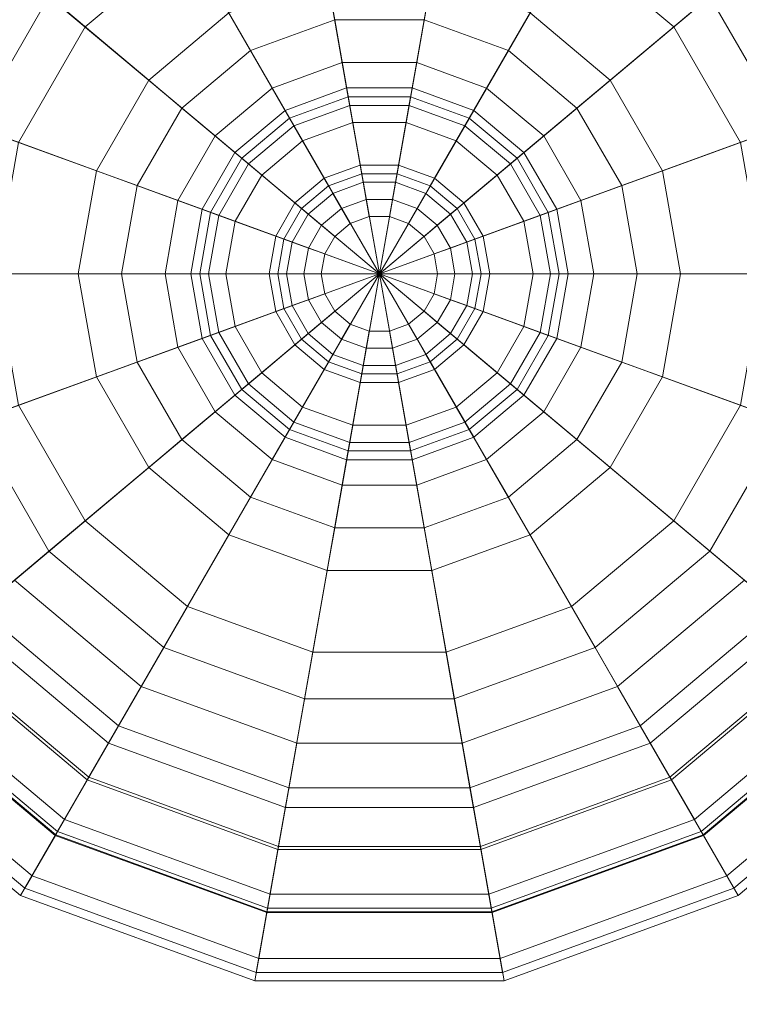
# Model space of a CAD drawing. Units: inches. Extents: x 375 to 1122, y 27 to 1069.
# Tile 58 of 155: x 732.383 to 733.741, y 305.711 to 307.569. Entities that reach past the tile are written whole.
import ezdxf

# ---------------------------------------------------------------- set-up
doc = ezdxf.new("R2010")
doc.units = ezdxf.units.IN
doc.layers.add('A-ANNO-DIMS', color=2, linetype='Continuous', lineweight=18)
doc.layers.add('Furniture', color=30, linetype='Continuous', lineweight=18)
doc.styles.get("Standard").update_dxf_attribs({"font": 'arial.ttf'})
doc.dimstyles.new('ISO-25', dxfattribs={"dimtxt": 12, "dimasz": 2.5, "dimexe": 1.5, "dimexo": 1.5, "dimtad": 1, "dimdec": 1, "dimlunit": 3, "dimtxsty": 'Standard', "dimblk": 'ARCHTICK', "dimcen": 2.5, "dimadec": 0, "dimazin": 0, "dimtfac": 1, "dimtdec": 1, "dimtmove": 0, "dimatfit": 3, "dimfxl": 1.5, "dimfxlon": 1, "dimarcsym": 0})

# ---------------------------------------------------------------- blocks, each defined once
blk = doc.blocks.new('A$C403C54AD')
for points in [[(0.980157, 1.23678, -0.04658), (0.980157, 1.202917, -0.043501), (0.980157, 1.202917, -0.043501), (0.968576, 1.234737, -0.04658)], [(0.991739, 1.234737, -0.04658), (0.980157, 1.202917, -0.043501), (0.980157, 1.202917, -0.043501), (0.980157, 1.23678, -0.04658)], [(0.968576, 1.234737, -0.04658), (0.980157, 1.202917, -0.043501), (0.980157, 1.202917, -0.043501), (0.958391, 1.228857, -0.04658)], [(1.001923, 1.228857, -0.04658), (0.980157, 1.202917, -0.043501), (0.980157, 1.202917, -0.043501), (0.991739, 1.234737, -0.04658)], [(0.980157, 1.217132, -0.040074), (0.980157, 1.233514, -0.043349), (0.969693, 1.231669, -0.043349), (0.975296, 1.216274, -0.040074)], [(0.985019, 1.216274, -0.040074), (0.990622, 1.231669, -0.043349), (0.980157, 1.233514, -0.043349), (0.980157, 1.217132, -0.040074)], [(0.975296, 1.216274, -0.040074), (0.969693, 1.231669, -0.043349), (0.96049, 1.226356, -0.043349), (0.971021, 1.213806, -0.040074)], [(0.989294, 1.213806, -0.040074), (0.999824, 1.226356, -0.043349), (0.990622, 1.231669, -0.043349), (0.985019, 1.216274, -0.040074)], [(0.958391, 1.228857, -0.04658), (0.980157, 1.202917, -0.043501), (0.980157, 1.202917, -0.043501), (0.950832, 1.219849, -0.04658)], [(0.970778, 1.228687, 0.056929), (0.973195, 1.222047, 0.046697), (0.967072, 1.218512, 0.046697), (0.96253, 1.223925, 0.056929)], [(1.009483, 1.219849, -0.04658), (0.980157, 1.202917, -0.043501), (0.980157, 1.202917, -0.043501), (1.001923, 1.228857, -0.04658)], [(0.997785, 1.223925, 0.056929), (0.993243, 1.218512, 0.046697), (0.98712, 1.222047, 0.046697), (0.989537, 1.228687, 0.056929)], [(1.00662, 1.218195, 0.116404), (1.009137, 1.219649, 0.10318), (1.001667, 1.228552, 0.10318), (0.999798, 1.226325, 0.116404)], [(1.006655, 1.218216, -0.043349), (1.009483, 1.219849, -0.04658), (1.001923, 1.228857, -0.04658), (0.999824, 1.226356, -0.043349)], [(1.009137, 1.219649, 0.10318), (1.008553, 1.219312, 0.074938), (1.001233, 1.228035, 0.074938), (1.001667, 1.228552, 0.10318)], [(1.008553, 1.219312, 0.074938), (1.003907, 1.216629, 0.056929), (0.997785, 1.223925, 0.056929), (1.001233, 1.228035, 0.074938)], [(0.971021, 1.213806, -0.040074), (0.96049, 1.226356, -0.043349), (0.95366, 1.218216, -0.043349), (0.967847, 1.210025, -0.040074)], [(0.992467, 1.210025, -0.040074), (1.006655, 1.218216, -0.043349), (0.999824, 1.226356, -0.043349), (0.989294, 1.213806, -0.040074)], [(1.002293, 1.215697, 0.12581), (1.00662, 1.218195, 0.116404), (0.999798, 1.226325, 0.116404), (0.996587, 1.222497, 0.12581)], [(0.973957, 1.219951, 0.048884), (0.971739, 1.226046, 0.058276), (0.964336, 1.221772, 0.058276), (0.968505, 1.216804, 0.048884)], [(0.991809, 1.216804, 0.048884), (0.995978, 1.221772, 0.058276), (0.988575, 1.226046, 0.058276), (0.986357, 1.219951, 0.048884)], [(1.006466, 1.218107, 0.102963), (1.004033, 1.216702, 0.115599), (0.997878, 1.224037, 0.115599), (0.999684, 1.226189, 0.102963)], [(1.005896, 1.217778, 0.075423), (1.006466, 1.218107, 0.102963), (0.999684, 1.226189, 0.102963), (0.999261, 1.225685, 0.075423)], [(1.001473, 1.215224, 0.058276), (1.005896, 1.217778, 0.075423), (0.999261, 1.225685, 0.075423), (0.995978, 1.221772, 0.058276)], [(1.003907, 1.216629, 0.056929), (0.997787, 1.213096, 0.046697), (0.993243, 1.218512, 0.046697), (0.997785, 1.223925, 0.056929)], [(1.004033, 1.216702, 0.115599), (0.999627, 1.214158, 0.12581), (0.994608, 1.220139, 0.12581), (0.997878, 1.224037, 0.115599)], [(0.980157, 1.223275, 0.046697), (0.980157, 1.213036, 0.03933), (0.976696, 1.212426, 0.03933), (0.973195, 1.222047, 0.046697)], [(0.98712, 1.222047, 0.046697), (0.983618, 1.212426, 0.03933), (0.980157, 1.213036, 0.03933), (0.980157, 1.223275, 0.046697)], [(0.973195, 1.222047, 0.046697), (0.976696, 1.212426, 0.03933), (0.973653, 1.210669, 0.03933), (0.967072, 1.218512, 0.046697)], [(0.993243, 1.218512, 0.046697), (0.986661, 1.210669, 0.03933), (0.983618, 1.212426, 0.03933), (0.98712, 1.222047, 0.046697)], [(0.999627, 1.214158, 0.12581), (1.002293, 1.215697, 0.12581), (0.996587, 1.222497, 0.12581), (0.994608, 1.220139, 0.12581)], [(0.968505, 1.216804, 0.048884), (0.964336, 1.221772, 0.058276), (0.958842, 1.215224, 0.058276), (0.964459, 1.211981, 0.048884)], [(0.995856, 1.211981, 0.048884), (1.001473, 1.215224, 0.058276), (0.995978, 1.221772, 0.058276), (0.991809, 1.216804, 0.048884)], [(0.980157, 1.211822, 0.042248), (0.980157, 1.221045, 0.048884), (0.973957, 1.219951, 0.048884), (0.977112, 1.211285, 0.042248)], [(0.983203, 1.211285, 0.042248), (0.986357, 1.219951, 0.048884), (0.980157, 1.221045, 0.048884), (0.980157, 1.211822, 0.042248)], [(0.950832, 1.219849, -0.04658), (0.980157, 1.202917, -0.043501), (0.980157, 1.202917, -0.043501), (0.94681, 1.208798, -0.04658)], [(0.977112, 1.211285, 0.042248), (0.973957, 1.219951, 0.048884), (0.968505, 1.216804, 0.048884), (0.974434, 1.209738, 0.042248)], [(1.013505, 1.208798, -0.04658), (0.980157, 1.202917, -0.043501), (0.980157, 1.202917, -0.043501), (1.009483, 1.219849, -0.04658)], [(0.985881, 1.209738, 0.042248), (0.991809, 1.216804, 0.048884), (0.986357, 1.219951, 0.048884), (0.983203, 1.211285, 0.042248)], [(1.010289, 1.20823, -0.043349), (1.013505, 1.208798, -0.04658), (1.009483, 1.219849, -0.04658), (1.006655, 1.218216, -0.043349)], [(1.012448, 1.208611, 0.074938), (1.007164, 1.20768, 0.056929), (1.003907, 1.216629, 0.056929), (1.008553, 1.219312, 0.074938)], [(1.010249, 1.208223, 0.116404), (1.013112, 1.208728, 0.10318), (1.009137, 1.219649, 0.10318), (1.00662, 1.218195, 0.116404)], [(1.013112, 1.208728, 0.10318), (1.012448, 1.208611, 0.074938), (1.008553, 1.219312, 0.074938), (1.009137, 1.219649, 0.10318)], [(0.967072, 1.218512, 0.046697), (0.973653, 1.210669, 0.03933), (0.971394, 1.207977, 0.03933), (0.962527, 1.213096, 0.046697)], [(0.997787, 1.213096, 0.046697), (0.98892, 1.207977, 0.03933), (0.986661, 1.210669, 0.03933), (0.993243, 1.218512, 0.046697)], [(0.994156, 1.205386, -0.040074), (1.010289, 1.20823, -0.043349), (1.006655, 1.218216, -0.043349), (0.992467, 1.210025, -0.040074)], [(1.005329, 1.207356, 0.12581), (1.010249, 1.208223, 0.116404), (1.00662, 1.218195, 0.116404), (1.002293, 1.215697, 0.12581)], [(1.010075, 1.208193, 0.102963), (1.007308, 1.207705, 0.115599), (1.004033, 1.216702, 0.115599), (1.006466, 1.218107, 0.102963)], [(1.009426, 1.208078, 0.075423), (1.010075, 1.208193, 0.102963), (1.006466, 1.218107, 0.102963), (1.005896, 1.217778, 0.075423)], [(1.004396, 1.207191, 0.058276), (1.009426, 1.208078, 0.075423), (1.005896, 1.217778, 0.075423), (1.001473, 1.215224, 0.058276)], [(0.980157, 1.215084, -0.037209), (0.980157, 1.217132, -0.040074), (0.975296, 1.216274, -0.040074), (0.975996, 1.21435, -0.037209)], [(0.984318, 1.21435, -0.037209), (0.985019, 1.216274, -0.040074), (0.980157, 1.217132, -0.040074), (0.980157, 1.215084, -0.037209)], [(0.974434, 1.209738, 0.042248), (0.968505, 1.216804, 0.048884), (0.964459, 1.211981, 0.048884), (0.972446, 1.207369, 0.042248)], [(0.987868, 1.207369, 0.042248), (0.995856, 1.211981, 0.048884), (0.991809, 1.216804, 0.048884), (0.985881, 1.209738, 0.042248)], [(1.007164, 1.20768, 0.056929), (1.000206, 1.206452, 0.046697), (0.997787, 1.213096, 0.046697), (1.003907, 1.216629, 0.056929)], [(1.007308, 1.207705, 0.115599), (1.002297, 1.206821, 0.12581), (0.999627, 1.214158, 0.12581), (1.004033, 1.216702, 0.115599)], [(0.975996, 1.21435, -0.037209), (0.975296, 1.216274, -0.040074), (0.971021, 1.213806, -0.040074), (0.972337, 1.212238, -0.037209)], [(0.987978, 1.212238, -0.037209), (0.989294, 1.213806, -0.040074), (0.985019, 1.216274, -0.040074), (0.984318, 1.21435, -0.037209)], [(1.002297, 1.206821, 0.12581), (1.005329, 1.207356, 0.12581), (1.002293, 1.215697, 0.12581), (0.999627, 1.214158, 0.12581)], [(0.980157, 1.210988, -0.035163), (0.980157, 1.215084, -0.037209), (0.975996, 1.21435, -0.037209), (0.977397, 1.210502, -0.035163)], [(0.982918, 1.210502, -0.035163), (0.984318, 1.21435, -0.037209), (0.980157, 1.215084, -0.037209), (0.980157, 1.210988, -0.035163)], [(0.998009, 1.206065, 0.048884), (1.004396, 1.207191, 0.058276), (1.001473, 1.215224, 0.058276), (0.995856, 1.211981, 0.048884)], [(0.977397, 1.210502, -0.035163), (0.975996, 1.21435, -0.037209), (0.972337, 1.212238, -0.037209), (0.974969, 1.2091, -0.035163)], [(0.985345, 1.2091, -0.035163), (0.987978, 1.212238, -0.037209), (0.984318, 1.21435, -0.037209), (0.982918, 1.210502, -0.035163)], [(0.972337, 1.212238, -0.037209), (0.971021, 1.213806, -0.040074), (0.967847, 1.210025, -0.040074), (0.969621, 1.209001, -0.037209)], [(0.990694, 1.209001, -0.037209), (0.992467, 1.210025, -0.040074), (0.989294, 1.213806, -0.040074), (0.987978, 1.212238, -0.037209)], [(0.962527, 1.213096, 0.046697), (0.971394, 1.207977, 0.03933), (0.970192, 1.204675, 0.03933), (0.960109, 1.206452, 0.046697)], [(0.980157, 1.213036, 0.03933), (0.980157, 1.208122, 0.038511), (0.978377, 1.207808, 0.038511), (0.976696, 1.212426, 0.03933)], [(0.983618, 1.212426, 0.03933), (0.981937, 1.207808, 0.038511), (0.980157, 1.208122, 0.038511), (0.980157, 1.213036, 0.03933)], [(1.000206, 1.206452, 0.046697), (0.990122, 1.204675, 0.03933), (0.98892, 1.207977, 0.03933), (0.997787, 1.213096, 0.046697)], [(0.976696, 1.212426, 0.03933), (0.978377, 1.207808, 0.038511), (0.976812, 1.206904, 0.038511), (0.973653, 1.210669, 0.03933)], [(0.986661, 1.210669, 0.03933), (0.983502, 1.206904, 0.038511), (0.981937, 1.207808, 0.038511), (0.983618, 1.212426, 0.03933)], [(0.972446, 1.207369, 0.042248), (0.964459, 1.211981, 0.048884), (0.962305, 1.206065, 0.048884), (0.971388, 1.204464, 0.042248)], [(0.974969, 1.2091, -0.035163), (0.972337, 1.212238, -0.037209), (0.969621, 1.209001, -0.037209), (0.973168, 1.206953, -0.035163)], [(0.980157, 1.202917, 0.040765), (0.980157, 1.211822, 0.042248), (0.977112, 1.211285, 0.042248), (0.980157, 1.202917, 0.040765)], [(0.980157, 1.202917, 0.040765), (0.983203, 1.211285, 0.042248), (0.980157, 1.211822, 0.042248), (0.980157, 1.202917, 0.040765)], [(0.987147, 1.206953, -0.035163), (0.990694, 1.209001, -0.037209), (0.987978, 1.212238, -0.037209), (0.985345, 1.2091, -0.035163)], [(0.988926, 1.204464, 0.042248), (0.998009, 1.206065, 0.048884), (0.995856, 1.211981, 0.048884), (0.987868, 1.207369, 0.042248)], [(0.980157, 1.211398, 0.035646), (0.980157, 1.207302, 0.033599), (0.978658, 1.207038, 0.033599), (0.977257, 1.210887, 0.035646)], [(0.980157, 1.210169, 0.037692), (0.980157, 1.211398, 0.035646), (0.977257, 1.210887, 0.035646), (0.977677, 1.209732, 0.037692)], [(0.983058, 1.210887, 0.035646), (0.981657, 1.207038, 0.033599), (0.980157, 1.207302, 0.033599), (0.980157, 1.211398, 0.035646)], [(0.982638, 1.209732, 0.037692), (0.983058, 1.210887, 0.035646), (0.980157, 1.211398, 0.035646), (0.980157, 1.210169, 0.037692)], [(0.980157, 1.202917, 0.040765), (0.977112, 1.211285, 0.042248), (0.974434, 1.209738, 0.042248), (0.980157, 1.202917, 0.040765)], [(0.980157, 1.207712, -0.029842), (0.980157, 1.210988, -0.035163), (0.977397, 1.210502, -0.035163), (0.978517, 1.207423, -0.029842)], [(0.980157, 1.202917, 0.040765), (0.985881, 1.209738, 0.042248), (0.983203, 1.211285, 0.042248), (0.980157, 1.202917, 0.040765)], [(0.981797, 1.207423, -0.029842), (0.982918, 1.210502, -0.035163), (0.980157, 1.210988, -0.035163), (0.980157, 1.207712, -0.029842)], [(0.973653, 1.210669, 0.03933), (0.976812, 1.206904, 0.038511), (0.97565, 1.205519, 0.038511), (0.971394, 1.207977, 0.03933)], [(0.977257, 1.210887, 0.035646), (0.978658, 1.207038, 0.033599), (0.977339, 1.206277, 0.033599), (0.974706, 1.209414, 0.035646)], [(0.977677, 1.209732, 0.037692), (0.977257, 1.210887, 0.035646), (0.974706, 1.209414, 0.035646), (0.975496, 1.208473, 0.037692)], [(0.978517, 1.207423, -0.029842), (0.977397, 1.210502, -0.035163), (0.974969, 1.2091, -0.035163), (0.977075, 1.20659, -0.029842)], [(0.985608, 1.209414, 0.035646), (0.982976, 1.206277, 0.033599), (0.981657, 1.207038, 0.033599), (0.983058, 1.210887, 0.035646)], [(0.983239, 1.20659, -0.029842), (0.985345, 1.2091, -0.035163), (0.982918, 1.210502, -0.035163), (0.981797, 1.207423, -0.029842)], [(0.984819, 1.208473, 0.037692), (0.985608, 1.209414, 0.035646), (0.983058, 1.210887, 0.035646), (0.982638, 1.209732, 0.037692)], [(0.98892, 1.207977, 0.03933), (0.984664, 1.205519, 0.038511), (0.983502, 1.206904, 0.038511), (0.986661, 1.210669, 0.03933)], [(0.969621, 1.209001, -0.037209), (0.967847, 1.210025, -0.040074), (0.966159, 1.205386, -0.040074), (0.968176, 1.20503, -0.037209)], [(0.980157, 1.208122, 0.038511), (0.980157, 1.210169, 0.037692), (0.977677, 1.209732, 0.037692), (0.978377, 1.207808, 0.038511)], [(0.981937, 1.207808, 0.038511), (0.982638, 1.209732, 0.037692), (0.980157, 1.210169, 0.037692), (0.980157, 1.208122, 0.038511)], [(0.992139, 1.20503, -0.037209), (0.994156, 1.205386, -0.040074), (0.992467, 1.210025, -0.040074), (0.990694, 1.209001, -0.037209)], [(0.980157, 1.202917, 0.040765), (0.974434, 1.209738, 0.042248), (0.972446, 1.207369, 0.042248), (0.980157, 1.202917, 0.040765)], [(0.978377, 1.207808, 0.038511), (0.977677, 1.209732, 0.037692), (0.975496, 1.208473, 0.037692), (0.976812, 1.206904, 0.038511)], [(0.980157, 1.202917, 0.040765), (0.987868, 1.207369, 0.042248), (0.985881, 1.209738, 0.042248), (0.980157, 1.202917, 0.040765)], [(0.983502, 1.206904, 0.038511), (0.984819, 1.208473, 0.037692), (0.982638, 1.209732, 0.037692), (0.981937, 1.207808, 0.038511)], [(0.974706, 1.209414, 0.035646), (0.977339, 1.206277, 0.033599), (0.97636, 1.20511, 0.033599), (0.972813, 1.207158, 0.035646)], [(0.975496, 1.208473, 0.037692), (0.974706, 1.209414, 0.035646), (0.972813, 1.207158, 0.035646), (0.973877, 1.206543, 0.037692)], [(0.977075, 1.20659, -0.029842), (0.974969, 1.2091, -0.035163), (0.973168, 1.206953, -0.035163), (0.976005, 1.205315, -0.029842)], [(0.987502, 1.207158, 0.035646), (0.983955, 1.20511, 0.033599), (0.982976, 1.206277, 0.033599), (0.985608, 1.209414, 0.035646)], [(0.98431, 1.205315, -0.029842), (0.987147, 1.206953, -0.035163), (0.985345, 1.2091, -0.035163), (0.983239, 1.20659, -0.029842)], [(0.986438, 1.206543, 0.037692), (0.987502, 1.207158, 0.035646), (0.985608, 1.209414, 0.035646), (0.984819, 1.208473, 0.037692)], [(0.94681, 1.208798, -0.04658), (0.980157, 1.202917, -0.043501), (0.980157, 1.202917, -0.043501), (0.94681, 1.197037, -0.04658)], [(0.973168, 1.206953, -0.035163), (0.969621, 1.209001, -0.037209), (0.968176, 1.20503, -0.037209), (0.972209, 1.204319, -0.035163)], [(1.013505, 1.197037, -0.04658), (0.980157, 1.202917, -0.043501), (0.980157, 1.202917, -0.043501), (1.013505, 1.208798, -0.04658)], [(0.988106, 1.204319, -0.035163), (0.992139, 1.20503, -0.037209), (0.990694, 1.209001, -0.037209), (0.987147, 1.206953, -0.035163)], [(1.012448, 1.197224, 0.074938), (1.007164, 1.198155, 0.056929), (1.007164, 1.20768, 0.056929), (1.012448, 1.208611, 0.074938)], [(1.010249, 1.197611, 0.116404), (1.013112, 1.197107, 0.10318), (1.013112, 1.208728, 0.10318), (1.010249, 1.208223, 0.116404)], [(1.010289, 1.197604, -0.043349), (1.013505, 1.197037, -0.04658), (1.013505, 1.208798, -0.04658), (1.010289, 1.20823, -0.043349)], [(1.013112, 1.197107, 0.10318), (1.012448, 1.197224, 0.074938), (1.012448, 1.208611, 0.074938), (1.013112, 1.208728, 0.10318)], [(0.976812, 1.206904, 0.038511), (0.975496, 1.208473, 0.037692), (0.973877, 1.206543, 0.037692), (0.97565, 1.205519, 0.038511)], [(0.984664, 1.205519, 0.038511), (0.986438, 1.206543, 0.037692), (0.984819, 1.208473, 0.037692), (0.983502, 1.206904, 0.038511)], [(0.994156, 1.200449, -0.040074), (1.010289, 1.197604, -0.043349), (1.010289, 1.20823, -0.043349), (0.994156, 1.205386, -0.040074)], [(1.005329, 1.198479, 0.12581), (1.010249, 1.197611, 0.116404), (1.010249, 1.208223, 0.116404), (1.005329, 1.207356, 0.12581)], [(1.010075, 1.197642, 0.102963), (1.007308, 1.19813, 0.115599), (1.007308, 1.207705, 0.115599), (1.010075, 1.208193, 0.102963)], [(1.009426, 1.197756, 0.075423), (1.010075, 1.197642, 0.102963), (1.010075, 1.208193, 0.102963), (1.009426, 1.208078, 0.075423)], [(0.971394, 1.207977, 0.03933), (0.97565, 1.205519, 0.038511), (0.975032, 1.203821, 0.038511), (0.970192, 1.204675, 0.03933)], [(0.980157, 1.206483, -0.021247), (0.980157, 1.207712, -0.029842), (0.978517, 1.207423, -0.029842), (0.978938, 1.206268, -0.021247)], [(0.981377, 1.206268, -0.021247), (0.981797, 1.207423, -0.029842), (0.980157, 1.207712, -0.029842), (0.980157, 1.206483, -0.021247)], [(0.990122, 1.204675, 0.03933), (0.985282, 1.203821, 0.038511), (0.984664, 1.205519, 0.038511), (0.98892, 1.207977, 0.03933)], [(1.007164, 1.198155, 0.056929), (1.000206, 1.199382, 0.046697), (1.000206, 1.206452, 0.046697), (1.007164, 1.20768, 0.056929)], [(1.007308, 1.19813, 0.115599), (1.002297, 1.199014, 0.12581), (1.002297, 1.206821, 0.12581), (1.007308, 1.207705, 0.115599)], [(1.004396, 1.198643, 0.058276), (1.009426, 1.197756, 0.075423), (1.009426, 1.208078, 0.075423), (1.004396, 1.207191, 0.058276)], [(0.980157, 1.202917, 0.040765), (0.972446, 1.207369, 0.042248), (0.971388, 1.204464, 0.042248), (0.980157, 1.202917, 0.040765)], [(0.978938, 1.206268, -0.021247), (0.978517, 1.207423, -0.029842), (0.977075, 1.20659, -0.029842), (0.977865, 1.205649, -0.021247)], [(0.980157, 1.207302, 0.033599), (0.980157, 1.205664, 0.027051), (0.979218, 1.205499, 0.027051), (0.978658, 1.207038, 0.033599)], [(0.980157, 1.202917, 0.040765), (0.988926, 1.204464, 0.042248), (0.987868, 1.207369, 0.042248), (0.980157, 1.202917, 0.040765)], [(0.981657, 1.207038, 0.033599), (0.981097, 1.205499, 0.027051), (0.980157, 1.205664, 0.027051), (0.980157, 1.207302, 0.033599)], [(0.982449, 1.205649, -0.021247), (0.983239, 1.20659, -0.029842), (0.981797, 1.207423, -0.029842), (0.981377, 1.206268, -0.021247)], [(0.998009, 1.19977, 0.048884), (1.004396, 1.198643, 0.058276), (1.004396, 1.207191, 0.058276), (0.998009, 1.206065, 0.048884)], [(1.002297, 1.199014, 0.12581), (1.005329, 1.198479, 0.12581), (1.005329, 1.207356, 0.12581), (1.002297, 1.206821, 0.12581)], [(0.972813, 1.207158, 0.035646), (0.97636, 1.20511, 0.033599), (0.975839, 1.203679, 0.033599), (0.971806, 1.20439, 0.035646)], [(0.973877, 1.206543, 0.037692), (0.972813, 1.207158, 0.035646), (0.971806, 1.20439, 0.035646), (0.973016, 1.204177, 0.037692)], [(0.976005, 1.205315, -0.029842), (0.973168, 1.206953, -0.035163), (0.972209, 1.204319, -0.035163), (0.975436, 1.20375, -0.029842)], [(0.978658, 1.207038, 0.033599), (0.979218, 1.205499, 0.027051), (0.978392, 1.205022, 0.027051), (0.977339, 1.206277, 0.033599)], [(0.982976, 1.206277, 0.033599), (0.981923, 1.205022, 0.027051), (0.981097, 1.205499, 0.027051), (0.981657, 1.207038, 0.033599)], [(0.988509, 1.20439, 0.035646), (0.984476, 1.203679, 0.033599), (0.983955, 1.20511, 0.033599), (0.987502, 1.207158, 0.035646)], [(0.984879, 1.20375, -0.029842), (0.988106, 1.204319, -0.035163), (0.987147, 1.206953, -0.035163), (0.98431, 1.205315, -0.029842)], [(0.987299, 1.204177, 0.037692), (0.988509, 1.20439, 0.035646), (0.987502, 1.207158, 0.035646), (0.986438, 1.206543, 0.037692)], [(0.960109, 1.206452, 0.046697), (0.970192, 1.204675, 0.03933), (0.970192, 1.20116, 0.03933), (0.960109, 1.199382, 0.046697)], [(0.97565, 1.205519, 0.038511), (0.973877, 1.206543, 0.037692), (0.973016, 1.204177, 0.037692), (0.975032, 1.203821, 0.038511)], [(0.977865, 1.205649, -0.021247), (0.977075, 1.20659, -0.029842), (0.976005, 1.205315, -0.029842), (0.977069, 1.2047, -0.021247)], [(0.977339, 1.206277, 0.033599), (0.978392, 1.205022, 0.027051), (0.977778, 1.204291, 0.027051), (0.97636, 1.20511, 0.033599)], [(0.979218, 1.205499, 0.027051), (0.978938, 1.206268, -0.021247), (0.977865, 1.205649, -0.021247), (0.978392, 1.205022, 0.027051)], [(0.980157, 1.205664, 0.027051), (0.980157, 1.206483, -0.021247), (0.978938, 1.206268, -0.021247), (0.979218, 1.205499, 0.027051)], [(0.981097, 1.205499, 0.027051), (0.981377, 1.206268, -0.021247), (0.980157, 1.206483, -0.021247), (0.980157, 1.205664, 0.027051)], [(0.981923, 1.205022, 0.027051), (0.982449, 1.205649, -0.021247), (0.981377, 1.206268, -0.021247), (0.981097, 1.205499, 0.027051)], [(0.983955, 1.20511, 0.033599), (0.982536, 1.204291, 0.027051), (0.981923, 1.205022, 0.027051), (0.982976, 1.206277, 0.033599)], [(0.983245, 1.2047, -0.021247), (0.98431, 1.205315, -0.029842), (0.983239, 1.20659, -0.029842), (0.982449, 1.205649, -0.021247)], [(0.985282, 1.203821, 0.038511), (0.987299, 1.204177, 0.037692), (0.986438, 1.206543, 0.037692), (0.984664, 1.205519, 0.038511)], [(1.000206, 1.199382, 0.046697), (0.990122, 1.20116, 0.03933), (0.990122, 1.204675, 0.03933), (1.000206, 1.206452, 0.046697)], [(0.971388, 1.204464, 0.042248), (0.962305, 1.206065, 0.048884), (0.962305, 1.19977, 0.048884), (0.971388, 1.201371, 0.042248)], [(0.988926, 1.201371, 0.042248), (0.998009, 1.19977, 0.048884), (0.998009, 1.206065, 0.048884), (0.988926, 1.204464, 0.042248)], [(0.968176, 1.20503, -0.037209), (0.966159, 1.205386, -0.040074), (0.966159, 1.200449, -0.040074), (0.968176, 1.200805, -0.037209)], [(0.977069, 1.2047, -0.021247), (0.976005, 1.205315, -0.029842), (0.975436, 1.20375, -0.029842), (0.976646, 1.203537, -0.021247)], [(0.978392, 1.205022, 0.027051), (0.977865, 1.205649, -0.021247), (0.977069, 1.2047, -0.021247), (0.977778, 1.204291, 0.027051)], [(0.982536, 1.204291, 0.027051), (0.983245, 1.2047, -0.021247), (0.982449, 1.205649, -0.021247), (0.981923, 1.205022, 0.027051)], [(0.983669, 1.203537, -0.021247), (0.984879, 1.20375, -0.029842), (0.98431, 1.205315, -0.029842), (0.983245, 1.2047, -0.021247)], [(0.992139, 1.200805, -0.037209), (0.994156, 1.200449, -0.040074), (0.994156, 1.205386, -0.040074), (0.992139, 1.20503, -0.037209)], [(0.972209, 1.204319, -0.035163), (0.968176, 1.20503, -0.037209), (0.968176, 1.200805, -0.037209), (0.972209, 1.201516, -0.035163)], [(0.97636, 1.20511, 0.033599), (0.977778, 1.204291, 0.027051), (0.977452, 1.203394, 0.027051), (0.975839, 1.203679, 0.033599)], [(0.984476, 1.203679, 0.033599), (0.982862, 1.203394, 0.027051), (0.982536, 1.204291, 0.027051), (0.983955, 1.20511, 0.033599)], [(0.988106, 1.201516, -0.035163), (0.992139, 1.200805, -0.037209), (0.992139, 1.20503, -0.037209), (0.988106, 1.204319, -0.035163)], [(0.970192, 1.204675, 0.03933), (0.975032, 1.203821, 0.038511), (0.975032, 1.202014, 0.038511), (0.970192, 1.20116, 0.03933)], [(0.980157, 1.202917, 0.040765), (0.971388, 1.204464, 0.042248), (0.971388, 1.201371, 0.042248), (0.980157, 1.202917, 0.040765)], [(0.971806, 1.20439, 0.035646), (0.975839, 1.203679, 0.033599), (0.975839, 1.202156, 0.033599), (0.971806, 1.201445, 0.035646)], [(0.973016, 1.204177, 0.037692), (0.971806, 1.20439, 0.035646), (0.971806, 1.201445, 0.035646), (0.973016, 1.201658, 0.037692)], [(0.977778, 1.204291, 0.027051), (0.977069, 1.2047, -0.021247), (0.976646, 1.203537, -0.021247), (0.977452, 1.203394, 0.027051)], [(0.980157, 1.202917, 0.040765), (0.988926, 1.201371, 0.042248), (0.988926, 1.204464, 0.042248), (0.980157, 1.202917, 0.040765)], [(0.982862, 1.203394, 0.027051), (0.983669, 1.203537, -0.021247), (0.983245, 1.2047, -0.021247), (0.982536, 1.204291, 0.027051)], [(0.988509, 1.201445, 0.035646), (0.984476, 1.202156, 0.033599), (0.984476, 1.203679, 0.033599), (0.988509, 1.20439, 0.035646)], [(0.990122, 1.20116, 0.03933), (0.985282, 1.202014, 0.038511), (0.985282, 1.203821, 0.038511), (0.990122, 1.204675, 0.03933)], [(0.987299, 1.201658, 0.037692), (0.988509, 1.201445, 0.035646), (0.988509, 1.20439, 0.035646), (0.987299, 1.204177, 0.037692)], [(0.975436, 1.20375, -0.029842), (0.972209, 1.204319, -0.035163), (0.972209, 1.201516, -0.035163), (0.975436, 1.202085, -0.029842)], [(0.975032, 1.203821, 0.038511), (0.973016, 1.204177, 0.037692), (0.973016, 1.201658, 0.037692), (0.975032, 1.202014, 0.038511)], [(0.984879, 1.202085, -0.029842), (0.988106, 1.201516, -0.035163), (0.988106, 1.204319, -0.035163), (0.984879, 1.20375, -0.029842)], [(0.985282, 1.202014, 0.038511), (0.987299, 1.201658, 0.037692), (0.987299, 1.204177, 0.037692), (0.985282, 1.203821, 0.038511)], [(0.976646, 1.203537, -0.021247), (0.975436, 1.20375, -0.029842), (0.975436, 1.202085, -0.029842), (0.976646, 1.202298, -0.021247)], [(0.975839, 1.203679, 0.033599), (0.977452, 1.203394, 0.027051), (0.977452, 1.20244, 0.027051), (0.975839, 1.202156, 0.033599)], [(0.977452, 1.203394, 0.027051), (0.976646, 1.203537, -0.021247), (0.976646, 1.202298, -0.021247), (0.977452, 1.20244, 0.027051)], [(0.984476, 1.202156, 0.033599), (0.982862, 1.20244, 0.027051), (0.982862, 1.203394, 0.027051), (0.984476, 1.203679, 0.033599)], [(0.982862, 1.20244, 0.027051), (0.983669, 1.202298, -0.021247), (0.983669, 1.203537, -0.021247), (0.982862, 1.203394, 0.027051)], [(0.983669, 1.202298, -0.021247), (0.984879, 1.202085, -0.029842), (0.984879, 1.20375, -0.029842), (0.983669, 1.203537, -0.021247)], [(0.94681, 1.197037, -0.04658), (0.980157, 1.202917, -0.043501), (0.980157, 1.202917, -0.043501), (0.950832, 1.185986, -0.04658)], [(0.950832, 1.185986, -0.04658), (0.980157, 1.202917, -0.043501), (0.980157, 1.202917, -0.043501), (0.958391, 1.176977, -0.04658)], [(0.958391, 1.176977, -0.04658), (0.980157, 1.202917, -0.043501), (0.980157, 1.202917, -0.043501), (0.968576, 1.171097, -0.04658)], [(0.968576, 1.171097, -0.04658), (0.980157, 1.202917, -0.043501), (0.980157, 1.202917, -0.043501), (0.980157, 1.169055, -0.04658)], [(0.980157, 1.202917, 0.040765), (0.971388, 1.201371, 0.042248), (0.972446, 1.198465, 0.042248), (0.980157, 1.202917, 0.040765)], [(0.980157, 1.202917, 0.040765), (0.972446, 1.198465, 0.042248), (0.974434, 1.196096, 0.042248), (0.980157, 1.202917, 0.040765)], [(0.980157, 1.202917, 0.040765), (0.974434, 1.196096, 0.042248), (0.977112, 1.19455, 0.042248), (0.980157, 1.202917, 0.040765)], [(0.980157, 1.202917, 0.040765), (0.977112, 1.19455, 0.042248), (0.980157, 1.194013, 0.042248), (0.980157, 1.202917, 0.040765)], [(0.980157, 1.202917, 0.040765), (0.983203, 1.19455, 0.042248), (0.985881, 1.196096, 0.042248), (0.980157, 1.202917, 0.040765)], [(0.980157, 1.202917, 0.040765), (0.980157, 1.194013, 0.042248), (0.983203, 1.19455, 0.042248), (0.980157, 1.202917, 0.040765)], [(0.980157, 1.202917, 0.040765), (0.987868, 1.198465, 0.042248), (0.988926, 1.201371, 0.042248), (0.980157, 1.202917, 0.040765)], [(0.980157, 1.202917, 0.040765), (0.985881, 1.196096, 0.042248), (0.987868, 1.198465, 0.042248), (0.980157, 1.202917, 0.040765)], [(1.009483, 1.185986, -0.04658), (0.980157, 1.202917, -0.043501), (0.980157, 1.202917, -0.043501), (1.013505, 1.197037, -0.04658)], [(1.001923, 1.176977, -0.04658), (0.980157, 1.202917, -0.043501), (0.980157, 1.202917, -0.043501), (1.009483, 1.185986, -0.04658)], [(0.991739, 1.171097, -0.04658), (0.980157, 1.202917, -0.043501), (0.980157, 1.202917, -0.043501), (1.001923, 1.176977, -0.04658)], [(0.980157, 1.169055, -0.04658), (0.980157, 1.202917, -0.043501), (0.980157, 1.202917, -0.043501), (0.991739, 1.171097, -0.04658)], [(0.971806, 1.201445, 0.035646), (0.975839, 1.202156, 0.033599), (0.97636, 1.200725, 0.033599), (0.972813, 1.198677, 0.035646)], [(0.975436, 1.202085, -0.029842), (0.972209, 1.201516, -0.035163), (0.973168, 1.198882, -0.035163), (0.976005, 1.20052, -0.029842)], [(0.976646, 1.202298, -0.021247), (0.975436, 1.202085, -0.029842), (0.976005, 1.20052, -0.029842), (0.977069, 1.201134, -0.021247)], [(0.975839, 1.202156, 0.033599), (0.977452, 1.20244, 0.027051), (0.977778, 1.201544, 0.027051), (0.97636, 1.200725, 0.033599)], [(0.977452, 1.20244, 0.027051), (0.976646, 1.202298, -0.021247), (0.977069, 1.201134, -0.021247), (0.977778, 1.201544, 0.027051)], [(0.983955, 1.200725, 0.033599), (0.982536, 1.201544, 0.027051), (0.982862, 1.20244, 0.027051), (0.984476, 1.202156, 0.033599)], [(0.982536, 1.201544, 0.027051), (0.983245, 1.201134, -0.021247), (0.983669, 1.202298, -0.021247), (0.982862, 1.20244, 0.027051)], [(0.983245, 1.201134, -0.021247), (0.98431, 1.20052, -0.029842), (0.984879, 1.202085, -0.029842), (0.983669, 1.202298, -0.021247)], [(0.987502, 1.198677, 0.035646), (0.983955, 1.200725, 0.033599), (0.984476, 1.202156, 0.033599), (0.988509, 1.201445, 0.035646)], [(0.98431, 1.20052, -0.029842), (0.987147, 1.198882, -0.035163), (0.988106, 1.201516, -0.035163), (0.984879, 1.202085, -0.029842)], [(0.970192, 1.20116, 0.03933), (0.975032, 1.202014, 0.038511), (0.97565, 1.200315, 0.038511), (0.971394, 1.197858, 0.03933)], [(0.973016, 1.201658, 0.037692), (0.971806, 1.201445, 0.035646), (0.972813, 1.198677, 0.035646), (0.973877, 1.199291, 0.037692)], [(0.975032, 1.202014, 0.038511), (0.973016, 1.201658, 0.037692), (0.973877, 1.199291, 0.037692), (0.97565, 1.200315, 0.038511)], [(0.984664, 1.200315, 0.038511), (0.986438, 1.199291, 0.037692), (0.987299, 1.201658, 0.037692), (0.985282, 1.202014, 0.038511)], [(0.98892, 1.197858, 0.03933), (0.984664, 1.200315, 0.038511), (0.985282, 1.202014, 0.038511), (0.990122, 1.20116, 0.03933)], [(0.986438, 1.199291, 0.037692), (0.987502, 1.198677, 0.035646), (0.988509, 1.201445, 0.035646), (0.987299, 1.201658, 0.037692)], [(0.960109, 1.199382, 0.046697), (0.970192, 1.20116, 0.03933), (0.971394, 1.197858, 0.03933), (0.962527, 1.192739, 0.046697)], [(0.971388, 1.201371, 0.042248), (0.962305, 1.19977, 0.048884), (0.964459, 1.193854, 0.048884), (0.972446, 1.198465, 0.042248)], [(0.972209, 1.201516, -0.035163), (0.968176, 1.200805, -0.037209), (0.969621, 1.196834, -0.037209), (0.973168, 1.198882, -0.035163)], [(0.977069, 1.201134, -0.021247), (0.976005, 1.20052, -0.029842), (0.977075, 1.199245, -0.029842), (0.977865, 1.200186, -0.021247)], [(0.97636, 1.200725, 0.033599), (0.977778, 1.201544, 0.027051), (0.978392, 1.200813, 0.027051), (0.977339, 1.199558, 0.033599)], [(0.977778, 1.201544, 0.027051), (0.977069, 1.201134, -0.021247), (0.977865, 1.200186, -0.021247), (0.978392, 1.200813, 0.027051)], [(0.982976, 1.199558, 0.033599), (0.981923, 1.200813, 0.027051), (0.982536, 1.201544, 0.027051), (0.983955, 1.200725, 0.033599)], [(0.981923, 1.200813, 0.027051), (0.982449, 1.200186, -0.021247), (0.983245, 1.201134, -0.021247), (0.982536, 1.201544, 0.027051)], [(0.982449, 1.200186, -0.021247), (0.983239, 1.199245, -0.029842), (0.98431, 1.20052, -0.029842), (0.983245, 1.201134, -0.021247)], [(0.987147, 1.198882, -0.035163), (0.990694, 1.196834, -0.037209), (0.992139, 1.200805, -0.037209), (0.988106, 1.201516, -0.035163)], [(0.987868, 1.198465, 0.042248), (0.995856, 1.193854, 0.048884), (0.998009, 1.19977, 0.048884), (0.988926, 1.201371, 0.042248)], [(0.997787, 1.192739, 0.046697), (0.98892, 1.197858, 0.03933), (0.990122, 1.20116, 0.03933), (1.000206, 1.199382, 0.046697)], [(0.968176, 1.200805, -0.037209), (0.966159, 1.200449, -0.040074), (0.967847, 1.19581, -0.040074), (0.969621, 1.196834, -0.037209)], [(0.972813, 1.198677, 0.035646), (0.97636, 1.200725, 0.033599), (0.977339, 1.199558, 0.033599), (0.974706, 1.196421, 0.035646)], [(0.977339, 1.199558, 0.033599), (0.978392, 1.200813, 0.027051), (0.979218, 1.200336, 0.027051), (0.978658, 1.198797, 0.033599)], [(0.978392, 1.200813, 0.027051), (0.977865, 1.200186, -0.021247), (0.978938, 1.199567, -0.021247), (0.979218, 1.200336, 0.027051)], [(0.981657, 1.198797, 0.033599), (0.981097, 1.200336, 0.027051), (0.981923, 1.200813, 0.027051), (0.982976, 1.199558, 0.033599)], [(0.981097, 1.200336, 0.027051), (0.981377, 1.199567, -0.021247), (0.982449, 1.200186, -0.021247), (0.981923, 1.200813, 0.027051)], [(0.985608, 1.196421, 0.035646), (0.982976, 1.199558, 0.033599), (0.983955, 1.200725, 0.033599), (0.987502, 1.198677, 0.035646)], [(0.990694, 1.196834, -0.037209), (0.992467, 1.19581, -0.040074), (0.994156, 1.200449, -0.040074), (0.992139, 1.200805, -0.037209)], [(0.971394, 1.197858, 0.03933), (0.97565, 1.200315, 0.038511), (0.976812, 1.198931, 0.038511), (0.973653, 1.195166, 0.03933)], [(0.976005, 1.20052, -0.029842), (0.973168, 1.198882, -0.035163), (0.974969, 1.196735, -0.035163), (0.977075, 1.199245, -0.029842)], [(0.97565, 1.200315, 0.038511), (0.973877, 1.199291, 0.037692), (0.975496, 1.197362, 0.037692), (0.976812, 1.198931, 0.038511)], [(0.978658, 1.198797, 0.033599), (0.979218, 1.200336, 0.027051), (0.980157, 1.200171, 0.027051), (0.980157, 1.198532, 0.033599)], [(0.979218, 1.200336, 0.027051), (0.978938, 1.199567, -0.021247), (0.980157, 1.199352, -0.021247), (0.980157, 1.200171, 0.027051)], [(0.980157, 1.198532, 0.033599), (0.980157, 1.200171, 0.027051), (0.981097, 1.200336, 0.027051), (0.981657, 1.198797, 0.033599)], [(0.980157, 1.200171, 0.027051), (0.980157, 1.199352, -0.021247), (0.981377, 1.199567, -0.021247), (0.981097, 1.200336, 0.027051)], [(0.983239, 1.199245, -0.029842), (0.985345, 1.196735, -0.035163), (0.987147, 1.198882, -0.035163), (0.98431, 1.20052, -0.029842)], [(0.983502, 1.198931, 0.038511), (0.984819, 1.197362, 0.037692), (0.986438, 1.199291, 0.037692), (0.984664, 1.200315, 0.038511)], [(0.986661, 1.195166, 0.03933), (0.983502, 1.198931, 0.038511), (0.984664, 1.200315, 0.038511), (0.98892, 1.197858, 0.03933)], [(0.992467, 1.19581, -0.040074), (1.006655, 1.187619, -0.043349), (1.010289, 1.197604, -0.043349), (0.994156, 1.200449, -0.040074)], [(0.977865, 1.200186, -0.021247), (0.977075, 1.199245, -0.029842), (0.978517, 1.198412, -0.029842), (0.978938, 1.199567, -0.021247)], [(0.981377, 1.199567, -0.021247), (0.981797, 1.198412, -0.029842), (0.983239, 1.199245, -0.029842), (0.982449, 1.200186, -0.021247)], [(0.995856, 1.193854, 0.048884), (1.001473, 1.190611, 0.058276), (1.004396, 1.198643, 0.058276), (0.998009, 1.19977, 0.048884)], [(0.973877, 1.199291, 0.037692), (0.972813, 1.198677, 0.035646), (0.974706, 1.196421, 0.035646), (0.975496, 1.197362, 0.037692)], [(0.974706, 1.196421, 0.035646), (0.977339, 1.199558, 0.033599), (0.978658, 1.198797, 0.033599), (0.977257, 1.194948, 0.035646)], [(0.978938, 1.199567, -0.021247), (0.978517, 1.198412, -0.029842), (0.980157, 1.198123, -0.029842), (0.980157, 1.199352, -0.021247)], [(0.980157, 1.199352, -0.021247), (0.980157, 1.198123, -0.029842), (0.981797, 1.198412, -0.029842), (0.981377, 1.199567, -0.021247)], [(0.983058, 1.194948, 0.035646), (0.981657, 1.198797, 0.033599), (0.982976, 1.199558, 0.033599), (0.985608, 1.196421, 0.035646)], [(0.984819, 1.197362, 0.037692), (0.985608, 1.196421, 0.035646), (0.987502, 1.198677, 0.035646), (0.986438, 1.199291, 0.037692)], [(1.003907, 1.189206, 0.056929), (0.997787, 1.192739, 0.046697), (1.000206, 1.199382, 0.046697), (1.007164, 1.198155, 0.056929)], [(0.973168, 1.198882, -0.035163), (0.969621, 1.196834, -0.037209), (0.972337, 1.193597, -0.037209), (0.974969, 1.196735, -0.035163)], [(0.973653, 1.195166, 0.03933), (0.976812, 1.198931, 0.038511), (0.978377, 1.198027, 0.038511), (0.976696, 1.193409, 0.03933)], [(0.977075, 1.199245, -0.029842), (0.974969, 1.196735, -0.035163), (0.977397, 1.195333, -0.035163), (0.978517, 1.198412, -0.029842)], [(0.976812, 1.198931, 0.038511), (0.975496, 1.197362, 0.037692), (0.977677, 1.196103, 0.037692), (0.978377, 1.198027, 0.038511)], [(0.981797, 1.198412, -0.029842), (0.982918, 1.195333, -0.035163), (0.985345, 1.196735, -0.035163), (0.983239, 1.199245, -0.029842)], [(0.981937, 1.198027, 0.038511), (0.982638, 1.196103, 0.037692), (0.984819, 1.197362, 0.037692), (0.983502, 1.198931, 0.038511)], [(0.983618, 1.193409, 0.03933), (0.981937, 1.198027, 0.038511), (0.983502, 1.198931, 0.038511), (0.986661, 1.195166, 0.03933)], [(0.985345, 1.196735, -0.035163), (0.987978, 1.193597, -0.037209), (0.990694, 1.196834, -0.037209), (0.987147, 1.198882, -0.035163)], [(0.999627, 1.191677, 0.12581), (1.002293, 1.190138, 0.12581), (1.005329, 1.198479, 0.12581), (1.002297, 1.199014, 0.12581)], [(1.004033, 1.189133, 0.115599), (0.999627, 1.191677, 0.12581), (1.002297, 1.199014, 0.12581), (1.007308, 1.19813, 0.115599)], [(0.972446, 1.198465, 0.042248), (0.964459, 1.193854, 0.048884), (0.968505, 1.189031, 0.048884), (0.974434, 1.196096, 0.042248)], [(0.977257, 1.194948, 0.035646), (0.978658, 1.198797, 0.033599), (0.980157, 1.198532, 0.033599), (0.980157, 1.194437, 0.035646)], [(0.978517, 1.198412, -0.029842), (0.977397, 1.195333, -0.035163), (0.980157, 1.194846, -0.035163), (0.980157, 1.198123, -0.029842)], [(0.980157, 1.194437, 0.035646), (0.980157, 1.198532, 0.033599), (0.981657, 1.198797, 0.033599), (0.983058, 1.194948, 0.035646)], [(0.980157, 1.198123, -0.029842), (0.980157, 1.194846, -0.035163), (0.982918, 1.195333, -0.035163), (0.981797, 1.198412, -0.029842)], [(0.985881, 1.196096, 0.042248), (0.991809, 1.189031, 0.048884), (0.995856, 1.193854, 0.048884), (0.987868, 1.198465, 0.042248)], [(1.001473, 1.190611, 0.058276), (1.005896, 1.188057, 0.075423), (1.009426, 1.197756, 0.075423), (1.004396, 1.198643, 0.058276)], [(1.002293, 1.190138, 0.12581), (1.00662, 1.187639, 0.116404), (1.010249, 1.197611, 0.116404), (1.005329, 1.198479, 0.12581)], [(0.976696, 1.193409, 0.03933), (0.978377, 1.198027, 0.038511), (0.980157, 1.197713, 0.038511), (0.980157, 1.192799, 0.03933)], [(0.978377, 1.198027, 0.038511), (0.977677, 1.196103, 0.037692), (0.980157, 1.195666, 0.037692), (0.980157, 1.197713, 0.038511)], [(0.980157, 1.197713, 0.038511), (0.980157, 1.195666, 0.037692), (0.982638, 1.196103, 0.037692), (0.981937, 1.198027, 0.038511)], [(0.980157, 1.192799, 0.03933), (0.980157, 1.197713, 0.038511), (0.981937, 1.198027, 0.038511), (0.983618, 1.193409, 0.03933)], [(1.008553, 1.186523, 0.074938), (1.003907, 1.189206, 0.056929), (1.007164, 1.198155, 0.056929), (1.012448, 1.197224, 0.074938)], [(1.006466, 1.187728, 0.102963), (1.004033, 1.189133, 0.115599), (1.007308, 1.19813, 0.115599), (1.010075, 1.197642, 0.102963)], [(0.962527, 1.192739, 0.046697), (0.971394, 1.197858, 0.03933), (0.973653, 1.195166, 0.03933), (0.967072, 1.187323, 0.046697)], [(0.993243, 1.187323, 0.046697), (0.986661, 1.195166, 0.03933), (0.98892, 1.197858, 0.03933), (0.997787, 1.192739, 0.046697)], [(1.005896, 1.188057, 0.075423), (1.006466, 1.187728, 0.102963), (1.010075, 1.197642, 0.102963), (1.009426, 1.197756, 0.075423)], [(1.00662, 1.187639, 0.116404), (1.009137, 1.186186, 0.10318), (1.013112, 1.197107, 0.10318), (1.010249, 1.197611, 0.116404)], [(1.006655, 1.187619, -0.043349), (1.009483, 1.185986, -0.04658), (1.013505, 1.197037, -0.04658), (1.010289, 1.197604, -0.043349)], [(0.975496, 1.197362, 0.037692), (0.974706, 1.196421, 0.035646), (0.977257, 1.194948, 0.035646), (0.977677, 1.196103, 0.037692)], [(0.982638, 1.196103, 0.037692), (0.983058, 1.194948, 0.035646), (0.985608, 1.196421, 0.035646), (0.984819, 1.197362, 0.037692)], [(1.009137, 1.186186, 0.10318), (1.008553, 1.186523, 0.074938), (1.012448, 1.197224, 0.074938), (1.013112, 1.197107, 0.10318)], [(0.969621, 1.196834, -0.037209), (0.967847, 1.19581, -0.040074), (0.971021, 1.192029, -0.040074), (0.972337, 1.193597, -0.037209)], [(0.974969, 1.196735, -0.035163), (0.972337, 1.193597, -0.037209), (0.975996, 1.191485, -0.037209), (0.977397, 1.195333, -0.035163)], [(0.982918, 1.195333, -0.035163), (0.984318, 1.191485, -0.037209), (0.987978, 1.193597, -0.037209), (0.985345, 1.196735, -0.035163)], [(0.987978, 1.193597, -0.037209), (0.989294, 1.192029, -0.040074), (0.992467, 1.19581, -0.040074), (0.990694, 1.196834, -0.037209)], [(0.974434, 1.196096, 0.042248), (0.968505, 1.189031, 0.048884), (0.973957, 1.185883, 0.048884), (0.977112, 1.19455, 0.042248)], [(0.977677, 1.196103, 0.037692), (0.977257, 1.194948, 0.035646), (0.980157, 1.194437, 0.035646), (0.980157, 1.195666, 0.037692)], [(0.980157, 1.195666, 0.037692), (0.980157, 1.194437, 0.035646), (0.983058, 1.194948, 0.035646), (0.982638, 1.196103, 0.037692)], [(0.983203, 1.19455, 0.042248), (0.986357, 1.185883, 0.048884), (0.991809, 1.189031, 0.048884), (0.985881, 1.196096, 0.042248)], [(0.967847, 1.19581, -0.040074), (0.95366, 1.187619, -0.043349), (0.96049, 1.179479, -0.043349), (0.971021, 1.192029, -0.040074)], [(0.989294, 1.192029, -0.040074), (0.999824, 1.179479, -0.043349), (1.006655, 1.187619, -0.043349), (0.992467, 1.19581, -0.040074)], [(0.967072, 1.187323, 0.046697), (0.973653, 1.195166, 0.03933), (0.976696, 1.193409, 0.03933), (0.973195, 1.183788, 0.046697)], [(0.977397, 1.195333, -0.035163), (0.975996, 1.191485, -0.037209), (0.980157, 1.190751, -0.037209), (0.980157, 1.194846, -0.035163)], [(0.980157, 1.194846, -0.035163), (0.980157, 1.190751, -0.037209), (0.984318, 1.191485, -0.037209), (0.982918, 1.195333, -0.035163)], [(0.98712, 1.183788, 0.046697), (0.983618, 1.193409, 0.03933), (0.986661, 1.195166, 0.03933), (0.993243, 1.187323, 0.046697)], [(0.977112, 1.19455, 0.042248), (0.973957, 1.185883, 0.048884), (0.980157, 1.18479, 0.048884), (0.980157, 1.194013, 0.042248)], [(0.980157, 1.194013, 0.042248), (0.980157, 1.18479, 0.048884), (0.986357, 1.185883, 0.048884), (0.983203, 1.19455, 0.042248)], [(0.964459, 1.193854, 0.048884), (0.958842, 1.190611, 0.058276), (0.964336, 1.184063, 0.058276), (0.968505, 1.189031, 0.048884)], [(0.991809, 1.189031, 0.048884), (0.995978, 1.184063, 0.058276), (1.001473, 1.190611, 0.058276), (0.995856, 1.193854, 0.048884)], [(0.972337, 1.193597, -0.037209), (0.971021, 1.192029, -0.040074), (0.975296, 1.18956, -0.040074), (0.975996, 1.191485, -0.037209)], [(0.973195, 1.183788, 0.046697), (0.976696, 1.193409, 0.03933), (0.980157, 1.192799, 0.03933), (0.980157, 1.18256, 0.046697)], [(0.980157, 1.18256, 0.046697), (0.980157, 1.192799, 0.03933), (0.983618, 1.193409, 0.03933), (0.98712, 1.183788, 0.046697)], [(0.984318, 1.191485, -0.037209), (0.985019, 1.18956, -0.040074), (0.989294, 1.192029, -0.040074), (0.987978, 1.193597, -0.037209)], [(0.997785, 1.18191, 0.056929), (0.993243, 1.187323, 0.046697), (0.997787, 1.192739, 0.046697), (1.003907, 1.189206, 0.056929)], [(0.971021, 1.192029, -0.040074), (0.96049, 1.179479, -0.043349), (0.969693, 1.174166, -0.043349), (0.975296, 1.18956, -0.040074)], [(0.985019, 1.18956, -0.040074), (0.990622, 1.174166, -0.043349), (0.999824, 1.179479, -0.043349), (0.989294, 1.192029, -0.040074)], [(0.975996, 1.191485, -0.037209), (0.975296, 1.18956, -0.040074), (0.980157, 1.188703, -0.040074), (0.980157, 1.190751, -0.037209)], [(0.980157, 1.190751, -0.037209), (0.980157, 1.188703, -0.040074), (0.985019, 1.18956, -0.040074), (0.984318, 1.191485, -0.037209)], [(0.994608, 1.185696, 0.12581), (0.996587, 1.183338, 0.12581), (1.002293, 1.190138, 0.12581), (0.999627, 1.191677, 0.12581)], [(0.997878, 1.181798, 0.115599), (0.994608, 1.185696, 0.12581), (0.999627, 1.191677, 0.12581), (1.004033, 1.189133, 0.115599)], [(0.995978, 1.184063, 0.058276), (0.999261, 1.18015, 0.075423), (1.005896, 1.188057, 0.075423), (1.001473, 1.190611, 0.058276)], [(0.996587, 1.183338, 0.12581), (0.999798, 1.17951, 0.116404), (1.00662, 1.187639, 0.116404), (1.002293, 1.190138, 0.12581)], [(0.975296, 1.18956, -0.040074), (0.969693, 1.174166, -0.043349), (0.980157, 1.172321, -0.043349), (0.980157, 1.188703, -0.040074)], [(0.980157, 1.188703, -0.040074), (0.980157, 1.172321, -0.043349), (0.990622, 1.174166, -0.043349), (0.985019, 1.18956, -0.040074)], [(1.001233, 1.1778, 0.074938), (0.997785, 1.18191, 0.056929), (1.003907, 1.189206, 0.056929), (1.008553, 1.186523, 0.074938)], [(0.999684, 1.179646, 0.102963), (0.997878, 1.181798, 0.115599), (1.004033, 1.189133, 0.115599), (1.006466, 1.187728, 0.102963)], [(0.968505, 1.189031, 0.048884), (0.964336, 1.184063, 0.058276), (0.971739, 1.179789, 0.058276), (0.973957, 1.185883, 0.048884)], [(0.986357, 1.185883, 0.048884), (0.988575, 1.179789, 0.058276), (0.995978, 1.184063, 0.058276), (0.991809, 1.189031, 0.048884)], [(0.999261, 1.18015, 0.075423), (0.999684, 1.179646, 0.102963), (1.006466, 1.187728, 0.102963), (1.005896, 1.188057, 0.075423)], [(0.96253, 1.18191, 0.056929), (0.967072, 1.187323, 0.046697), (0.973195, 1.183788, 0.046697), (0.970778, 1.177147, 0.056929)], [(0.989537, 1.177147, 0.056929), (0.98712, 1.183788, 0.046697), (0.993243, 1.187323, 0.046697), (0.997785, 1.18191, 0.056929)], [(0.999798, 1.17951, 0.116404), (1.001667, 1.177283, 0.10318), (1.009137, 1.186186, 0.10318), (1.00662, 1.187639, 0.116404)], [(0.999824, 1.179479, -0.043349), (1.001923, 1.176977, -0.04658), (1.009483, 1.185986, -0.04658), (1.006655, 1.187619, -0.043349)], [(1.001667, 1.177283, 0.10318), (1.001233, 1.1778, 0.074938), (1.008553, 1.186523, 0.074938), (1.009137, 1.186186, 0.10318)]]:
    blk.add_3dface(points)
blk = doc.blocks.new('_ArchTick')
at = {"color": 0, "linetype": 'ByBlock', "const_width": 0.15}
blk.add_lwpolyline([(-0.5, -0.5), (0.5, 0.5)], dxfattribs=at)
blk = doc.blocks.new('*D94')
at = {"layer": 'A-ANNO-DIMS', "color": 0, "lineweight": -2, "transparency": 16777216}
for p, q in [((734.0073, 117.5277), (734.0073, 114.5277)), ((773.0073, 117.5277), (773.0073, 114.5277)), ((734.0073, 116.0277), (773.0073, 116.0277))]:
    blk.add_line(p, q, dxfattribs=at)
at = {"layer": 'Defpoints', "color": 0, "transparency": 16777216}
for p in [(734.0073, 667.5277), (773.0073, 667.5277), (773.0073, 116.0277)]:
    blk.add_point(p, dxfattribs=at)
at = {"layer": 'A-ANNO-DIMS', "color": 0, "lineweight": -2, "transparency": 16777216, "xscale": 2.5, "yscale": 2.5, "zscale": 2.5, "rotation": 180}
blk.add_blockref('_ArchTick', (734.0073, 116.0277), dxfattribs=at)
at = {"layer": 'A-ANNO-DIMS', "color": 0, "lineweight": -2, "transparency": 16777216, "xscale": 2.5, "yscale": 2.5, "zscale": 2.5}
blk.add_blockref('_ArchTick', (773.0073, 116.0277), dxfattribs=at)
at = {"layer": 'A-ANNO-DIMS', "color": 0, "transparency": 16777216, "insert": (753.5073, 122.7837), "char_height": 12, "attachment_point": 5}
blk.add_mtext('3\'-3"', dxfattribs=at)

msp = doc.modelspace()

# ---------------------------------------------------------------- block references
at = {"layer": 'Furniture', "xscale": 39.9918517141215, "yscale": 39.9918517141215, "zscale": 39.9918517141215, "rotation": 270}
msp.add_blockref('A$C403C54AD', (684.9549, 346.2875, 0.024), dxfattribs=at)

# ---------------------------------------------------------------- dimensions: what is measured, and where the dimension line sits
at = {"layer": 'A-ANNO-DIMS'}
dim = msp.add_linear_dim(base=(773.0073, 116.0277), p1=(734.0073, 667.5277), p2=(773.0073, 667.5277), dimstyle='ISO-25', override={"dimdec": 1, "dimlfac": 1, "dimrnd": 0, "dimzin": 1, "dimdsep": 46, "dimlunit": 4, "dimfrac": 2}, dxfattribs=at)
dim.commit()
dim.dimension.update_dxf_attribs({"geometry": '*D94', "text_midpoint": (753.5073, 122.7837)})

doc.saveas('drawing.dxf')
